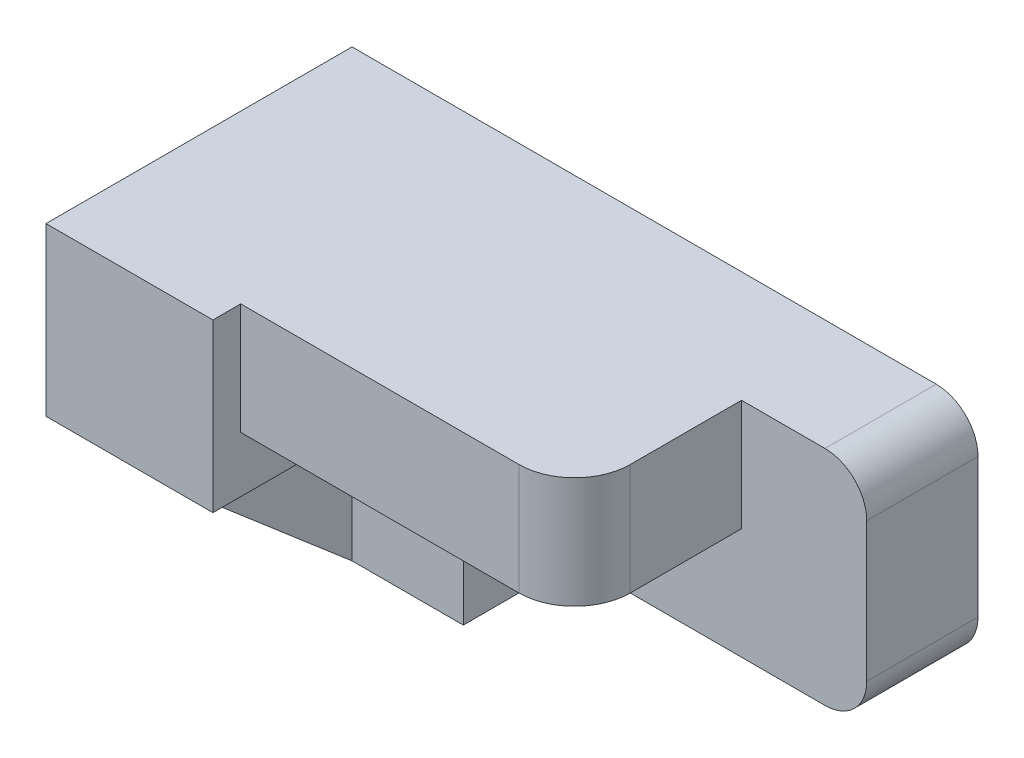
ISO-10303-21;
HEADER;
FILE_DESCRIPTION(('STEP AP214'),'2;1');
FILE_NAME('part.step','',(''),(''),'','','');
FILE_SCHEMA(('AUTOMOTIVE_DESIGN { 1 0 10303 214 1 1 1 1 }'));
ENDSEC;
DATA;
#1=APPLICATION_CONTEXT('core data for automotive mechanical design processes');
#2=APPLICATION_PROTOCOL_DEFINITION('international standard','automotive_design',2000,#1);
#3=PRODUCT_CONTEXT('',#1,'mechanical');
#4=PRODUCT('Part','Part','',(#3));
#5=PRODUCT_RELATED_PRODUCT_CATEGORY('part','',(#4));
#6=PRODUCT_DEFINITION_FORMATION('','',#4);
#7=PRODUCT_DEFINITION_CONTEXT('part definition',#1,'design');
#8=PRODUCT_DEFINITION('design','',#6,#7);
#9=PRODUCT_DEFINITION_SHAPE('','',#8);
#10=(LENGTH_UNIT() NAMED_UNIT(*) SI_UNIT(.MILLI.,.METRE.));
#11=(NAMED_UNIT(*) PLANE_ANGLE_UNIT() SI_UNIT($,.RADIAN.));
#12=(NAMED_UNIT(*) SI_UNIT($,.STERADIAN.) SOLID_ANGLE_UNIT());
#13=UNCERTAINTY_MEASURE_WITH_UNIT(LENGTH_MEASURE(1.E-05),#10,'distance_accuracy_value','');
#14=(GEOMETRIC_REPRESENTATION_CONTEXT(3) GLOBAL_UNCERTAINTY_ASSIGNED_CONTEXT((#13)) GLOBAL_UNIT_ASSIGNED_CONTEXT((#10,
#11,#12)) REPRESENTATION_CONTEXT('',''));
#15=CARTESIAN_POINT('',(0.,0.,0.));
#16=DIRECTION('',(0.,0.,1.));
#17=DIRECTION('',(1.,0.,0.));
#18=AXIS2_PLACEMENT_3D('',#15,#16,#17);
#19=CARTESIAN_POINT('',(20.,10.,55.));
#20=DIRECTION('',(0.,-0.759256602365297,0.650791373455968));
#21=DIRECTION('',(0.,-0.650791373455968,-0.759256602365297));
#22=AXIS2_PLACEMENT_3D('',#19,#20,#21);
#23=PLANE('',#22);
#24=DIRECTION('',(1.,0.,0.));
#25=VECTOR('',#24,1.);
#26=CARTESIAN_POINT('',(30.,10.,55.));
#27=LINE('',#26,#25);
#28=CARTESIAN_POINT('',(12.,10.,55.));
#29=VERTEX_POINT('',#28);
#30=CARTESIAN_POINT('',(20.,10.,55.));
#31=VERTEX_POINT('',#30);
#32=EDGE_CURVE('E68',#29,#31,#27,.T.);
#33=ORIENTED_EDGE('',*,*,#32,.F.);
#34=DIRECTION('',(0.,0.650791373455969,0.759256602365297));
#35=VECTOR('',#34,1.);
#36=CARTESIAN_POINT('',(12.,10.,55.));
#37=LINE('',#36,#35);
#38=CARTESIAN_POINT('',(12.,-20.,20.));
#39=VERTEX_POINT('',#38);
#40=EDGE_CURVE('E185',#39,#29,#37,.T.);
#41=ORIENTED_EDGE('',*,*,#40,.F.);
#42=DIRECTION('',(-1.,0.,0.));
#43=VECTOR('',#42,1.);
#44=CARTESIAN_POINT('',(20.,-20.,20.));
#45=LINE('',#44,#43);
#46=CARTESIAN_POINT('',(20.,-20.,20.));
#47=VERTEX_POINT('',#46);
#48=EDGE_CURVE('E202',#47,#39,#45,.T.);
#49=ORIENTED_EDGE('',*,*,#48,.F.);
#50=DIRECTION('',(0.,0.650791373455969,0.759256602365297));
#51=VECTOR('',#50,1.);
#52=CARTESIAN_POINT('',(20.,10.,55.));
#53=LINE('',#52,#51);
#54=EDGE_CURVE('E200',#47,#31,#53,.T.);
#55=ORIENTED_EDGE('',*,*,#54,.T.);
#56=EDGE_LOOP('',(#33,#41,#49,#55));
#57=FACE_BOUND('',#56,.T.);
#58=ADVANCED_FACE('F50',(#57),#23,.T.);
#59=CARTESIAN_POINT('',(105.,7.5,20.));
#60=DIRECTION('',(0.,0.,1.));
#61=DIRECTION('',(1.,0.,0.));
#62=AXIS2_PLACEMENT_3D('',#59,#60,#61);
#63=PLANE('',#62);
#64=DIRECTION('',(0.,-1.,0.));
#65=VECTOR('',#64,1.);
#66=CARTESIAN_POINT('',(20.,-20.,20.));
#67=LINE('',#66,#65);
#68=CARTESIAN_POINT('',(20.,10.,20.));
#69=VERTEX_POINT('',#68);
#70=EDGE_CURVE('E193',#69,#47,#67,.T.);
#71=ORIENTED_EDGE('',*,*,#70,.T.);
#72=DIRECTION('',(-1.,0.,0.));
#73=VECTOR('',#72,1.);
#74=CARTESIAN_POINT('',(0.,-20.,20.));
#75=LINE('',#74,#73);
#76=CARTESIAN_POINT('',(40.,-20.,20.));
#77=VERTEX_POINT('',#76);
#78=EDGE_CURVE('E268',#77,#47,#75,.T.);
#79=ORIENTED_EDGE('',*,*,#78,.F.);
#80=DIRECTION('',(0.,1.,0.));
#81=VECTOR('',#80,1.);
#82=CARTESIAN_POINT('',(40.,-20.,20.));
#83=LINE('',#82,#81);
#84=CARTESIAN_POINT('',(40.,0.,20.));
#85=VERTEX_POINT('',#84);
#86=EDGE_CURVE('E271',#77,#85,#83,.T.);
#87=ORIENTED_EDGE('',*,*,#86,.T.);
#88=DIRECTION('',(1.,0.,0.));
#89=VECTOR('',#88,1.);
#90=CARTESIAN_POINT('',(0.,0.,20.));
#91=LINE('',#90,#89);
#92=CARTESIAN_POINT('',(105.,0.,20.));
#93=VERTEX_POINT('',#92);
#94=EDGE_CURVE('E278',#85,#93,#91,.T.);
#95=ORIENTED_EDGE('',*,*,#94,.T.);
#96=CARTESIAN_POINT('',(105.,7.5,20.));
#97=DIRECTION('',(0.,0.,1.));
#98=DIRECTION('',(1.,0.,0.));
#99=AXIS2_PLACEMENT_3D('',#96,#97,#98);
#100=CIRCLE('',#99,7.5);
#101=CARTESIAN_POINT('',(112.5,7.5,20.));
#102=VERTEX_POINT('',#101);
#103=EDGE_CURVE('E285',#93,#102,#100,.T.);
#104=ORIENTED_EDGE('',*,*,#103,.T.);
#105=DIRECTION('',(0.,1.,0.));
#106=VECTOR('',#105,1.);
#107=CARTESIAN_POINT('',(112.5,32.5,20.));
#108=LINE('',#107,#106);
#109=CARTESIAN_POINT('',(112.5,32.5,20.));
#110=VERTEX_POINT('',#109);
#111=EDGE_CURVE('E281',#102,#110,#108,.T.);
#112=ORIENTED_EDGE('',*,*,#111,.T.);
#113=CARTESIAN_POINT('',(105.,32.5,20.));
#114=DIRECTION('',(0.,0.,1.));
#115=DIRECTION('',(1.,0.,0.));
#116=AXIS2_PLACEMENT_3D('',#113,#114,#115);
#117=CIRCLE('',#116,7.5);
#118=CARTESIAN_POINT('',(105.,40.,20.));
#119=VERTEX_POINT('',#118);
#120=EDGE_CURVE('E289',#110,#119,#117,.T.);
#121=ORIENTED_EDGE('',*,*,#120,.T.);
#122=DIRECTION('',(-1.,0.,0.));
#123=VECTOR('',#122,1.);
#124=CARTESIAN_POINT('',(0.,40.,20.));
#125=LINE('',#124,#123);
#126=CARTESIAN_POINT('',(90.,40.,20.));
#127=VERTEX_POINT('',#126);
#128=EDGE_CURVE('E286',#119,#127,#125,.T.);
#129=ORIENTED_EDGE('',*,*,#128,.T.);
#130=DIRECTION('',(0.,1.,0.));
#131=VECTOR('',#130,1.);
#132=CARTESIAN_POINT('',(90.,20.,20.));
#133=LINE('',#132,#131);
#134=CARTESIAN_POINT('',(90.,20.,20.));
#135=VERTEX_POINT('',#134);
#136=EDGE_CURVE('E231',#135,#127,#133,.T.);
#137=ORIENTED_EDGE('',*,*,#136,.F.);
#138=DIRECTION('',(1.,0.,0.));
#139=VECTOR('',#138,1.);
#140=CARTESIAN_POINT('',(0.,20.,20.));
#141=LINE('',#140,#139);
#142=CARTESIAN_POINT('',(30.,20.,20.));
#143=VERTEX_POINT('',#142);
#144=EDGE_CURVE('E217',#143,#135,#141,.T.);
#145=ORIENTED_EDGE('',*,*,#144,.F.);
#146=DIRECTION('',(0.,1.,0.));
#147=VECTOR('',#146,1.);
#148=CARTESIAN_POINT('',(30.,40.,20.));
#149=LINE('',#148,#147);
#150=CARTESIAN_POINT('',(30.,10.,20.));
#151=VERTEX_POINT('',#150);
#152=EDGE_CURVE('E243',#151,#143,#149,.T.);
#153=ORIENTED_EDGE('',*,*,#152,.F.);
#154=DIRECTION('',(1.,0.,0.));
#155=VECTOR('',#154,1.);
#156=CARTESIAN_POINT('',(30.,10.,20.));
#157=LINE('',#156,#155);
#158=EDGE_CURVE('E235',#69,#151,#157,.T.);
#159=ORIENTED_EDGE('',*,*,#158,.F.);
#160=EDGE_LOOP('',(#71,#79,#87,#95,#104,#112,#121,#129,#137,#145,#153,#159));
#161=FACE_BOUND('',#160,.T.);
#162=ADVANCED_FACE('F333',(#161),#63,.T.);
#163=CARTESIAN_POINT('',(0.,0.,20.));
#164=DIRECTION('',(0.,1.,0.));
#165=DIRECTION('',(0.,0.,1.));
#166=AXIS2_PLACEMENT_3D('',#163,#164,#165);
#167=PLANE('',#166);
#168=DIRECTION('',(0.,0.,1.));
#169=VECTOR('',#168,1.);
#170=CARTESIAN_POINT('',(40.,0.,20.));
#171=LINE('',#170,#169);
#172=CARTESIAN_POINT('',(40.,0.,0.));
#173=VERTEX_POINT('',#172);
#174=EDGE_CURVE('E257',#173,#85,#171,.T.);
#175=ORIENTED_EDGE('',*,*,#174,.F.);
#176=DIRECTION('',(1.,0.,0.));
#177=VECTOR('',#176,1.);
#178=CARTESIAN_POINT('',(0.,0.,0.));
#179=LINE('',#178,#177);
#180=CARTESIAN_POINT('',(105.,0.,0.));
#181=VERTEX_POINT('',#180);
#182=EDGE_CURVE('E294',#173,#181,#179,.T.);
#183=ORIENTED_EDGE('',*,*,#182,.T.);
#184=DIRECTION('',(0.,0.,-1.));
#185=VECTOR('',#184,1.);
#186=CARTESIAN_POINT('',(105.,0.,20.));
#187=LINE('',#186,#185);
#188=EDGE_CURVE('E11',#93,#181,#187,.T.);
#189=ORIENTED_EDGE('',*,*,#188,.F.);
#190=ORIENTED_EDGE('',*,*,#94,.F.);
#191=EDGE_LOOP('',(#175,#183,#189,#190));
#192=FACE_BOUND('',#191,.T.);
#193=ADVANCED_FACE('F342',(#192),#167,.F.);
#194=CARTESIAN_POINT('',(0.,40.,20.));
#195=DIRECTION('',(1.,0.,0.));
#196=DIRECTION('',(0.,0.,-1.));
#197=AXIS2_PLACEMENT_3D('',#194,#195,#196);
#198=PLANE('',#197);
#199=DIRECTION('',(0.,-1.,0.));
#200=VECTOR('',#199,1.);
#201=CARTESIAN_POINT('',(0.,-20.,20.));
#202=LINE('',#201,#200);
#203=CARTESIAN_POINT('',(0.,10.,20.));
#204=VERTEX_POINT('',#203);
#205=CARTESIAN_POINT('',(0.,-20.,20.));
#206=VERTEX_POINT('',#205);
#207=EDGE_CURVE('E189',#204,#206,#202,.T.);
#208=ORIENTED_EDGE('',*,*,#207,.F.);
#209=DIRECTION('',(0.,0.,-1.));
#210=VECTOR('',#209,1.);
#211=CARTESIAN_POINT('',(0.,10.,20.));
#212=LINE('',#211,#210);
#213=CARTESIAN_POINT('',(0.,10.,55.));
#214=VERTEX_POINT('',#213);
#215=EDGE_CURVE('E180',#214,#204,#212,.T.);
#216=ORIENTED_EDGE('',*,*,#215,.F.);
#217=DIRECTION('',(0.,-1.,0.));
#218=VECTOR('',#217,1.);
#219=CARTESIAN_POINT('',(0.,10.,55.));
#220=LINE('',#219,#218);
#221=CARTESIAN_POINT('',(0.,40.,55.));
#222=VERTEX_POINT('',#221);
#223=EDGE_CURVE('E239',#222,#214,#220,.T.);
#224=ORIENTED_EDGE('',*,*,#223,.F.);
#225=DIRECTION('',(0.,0.,-1.));
#226=VECTOR('',#225,1.);
#227=CARTESIAN_POINT('',(0.,40.,20.));
#228=LINE('',#227,#226);
#229=CARTESIAN_POINT('',(0.,40.,0.));
#230=VERTEX_POINT('',#229);
#231=EDGE_CURVE('E295',#222,#230,#228,.T.);
#232=ORIENTED_EDGE('',*,*,#231,.T.);
#233=DIRECTION('',(0.,-1.,0.));
#234=VECTOR('',#233,1.);
#235=CARTESIAN_POINT('',(0.,40.,0.));
#236=LINE('',#235,#234);
#237=CARTESIAN_POINT('',(0.,-20.,0.));
#238=VERTEX_POINT('',#237);
#239=EDGE_CURVE('E276',#230,#238,#236,.T.);
#240=ORIENTED_EDGE('',*,*,#239,.T.);
#241=DIRECTION('',(0.,0.,-1.));
#242=VECTOR('',#241,1.);
#243=CARTESIAN_POINT('',(0.,-20.,0.));
#244=LINE('',#243,#242);
#245=EDGE_CURVE('E261',#206,#238,#244,.T.);
#246=ORIENTED_EDGE('',*,*,#245,.F.);
#247=EDGE_LOOP('',(#208,#216,#224,#232,#240,#246));
#248=FACE_BOUND('',#247,.T.);
#249=ADVANCED_FACE('F47',(#248),#198,.F.);
#250=CARTESIAN_POINT('',(105.,7.5,20.));
#251=DIRECTION('',(0.,0.,-1.));
#252=DIRECTION('',(-1.,0.,0.));
#253=AXIS2_PLACEMENT_3D('',#250,#251,#252);
#254=CYLINDRICAL_SURFACE('',#253,7.5);
#255=CARTESIAN_POINT('',(105.,7.5,0.));
#256=DIRECTION('',(0.,0.,1.));
#257=DIRECTION('',(1.,0.,0.));
#258=AXIS2_PLACEMENT_3D('',#255,#256,#257);
#259=CIRCLE('',#258,7.5);
#260=CARTESIAN_POINT('',(112.5,7.5,0.));
#261=VERTEX_POINT('',#260);
#262=EDGE_CURVE('E297',#181,#261,#259,.T.);
#263=ORIENTED_EDGE('',*,*,#262,.T.);
#264=DIRECTION('',(0.,0.,-1.));
#265=VECTOR('',#264,1.);
#266=CARTESIAN_POINT('',(112.5,7.5,20.));
#267=LINE('',#266,#265);
#268=EDGE_CURVE('E54',#102,#261,#267,.T.);
#269=ORIENTED_EDGE('',*,*,#268,.F.);
#270=ORIENTED_EDGE('',*,*,#103,.F.);
#271=ORIENTED_EDGE('',*,*,#188,.T.);
#272=EDGE_LOOP('',(#263,#269,#270,#271));
#273=FACE_BOUND('',#272,.T.);
#274=ADVANCED_FACE('F338',(#273),#254,.T.);
#275=CARTESIAN_POINT('',(112.5,32.5,20.));
#276=DIRECTION('',(-1.,0.,0.));
#277=DIRECTION('',(0.,0.,1.));
#278=AXIS2_PLACEMENT_3D('',#275,#276,#277);
#279=PLANE('',#278);
#280=DIRECTION('',(0.,1.,0.));
#281=VECTOR('',#280,1.);
#282=CARTESIAN_POINT('',(112.5,32.5,0.));
#283=LINE('',#282,#281);
#284=CARTESIAN_POINT('',(112.5,32.5,0.));
#285=VERTEX_POINT('',#284);
#286=EDGE_CURVE('E298',#261,#285,#283,.T.);
#287=ORIENTED_EDGE('',*,*,#286,.T.);
#288=DIRECTION('',(0.,0.,-1.));
#289=VECTOR('',#288,1.);
#290=CARTESIAN_POINT('',(112.5,32.5,20.));
#291=LINE('',#290,#289);
#292=EDGE_CURVE('E306',#110,#285,#291,.T.);
#293=ORIENTED_EDGE('',*,*,#292,.F.);
#294=ORIENTED_EDGE('',*,*,#111,.F.);
#295=ORIENTED_EDGE('',*,*,#268,.T.);
#296=EDGE_LOOP('',(#287,#293,#294,#295));
#297=FACE_BOUND('',#296,.T.);
#298=ADVANCED_FACE('F312',(#297),#279,.F.);
#299=CARTESIAN_POINT('',(105.,32.5,20.));
#300=DIRECTION('',(0.,0.,-1.));
#301=DIRECTION('',(-1.,0.,0.));
#302=AXIS2_PLACEMENT_3D('',#299,#300,#301);
#303=CYLINDRICAL_SURFACE('',#302,7.5);
#304=CARTESIAN_POINT('',(105.,32.5,0.));
#305=DIRECTION('',(0.,0.,1.));
#306=DIRECTION('',(1.,0.,0.));
#307=AXIS2_PLACEMENT_3D('',#304,#305,#306);
#308=CIRCLE('',#307,7.5);
#309=CARTESIAN_POINT('',(105.,40.,0.));
#310=VERTEX_POINT('',#309);
#311=EDGE_CURVE('E296',#285,#310,#308,.T.);
#312=ORIENTED_EDGE('',*,*,#311,.T.);
#313=DIRECTION('',(0.,0.,-1.));
#314=VECTOR('',#313,1.);
#315=CARTESIAN_POINT('',(105.,40.,20.));
#316=LINE('',#315,#314);
#317=EDGE_CURVE('E303',#119,#310,#316,.T.);
#318=ORIENTED_EDGE('',*,*,#317,.F.);
#319=ORIENTED_EDGE('',*,*,#120,.F.);
#320=ORIENTED_EDGE('',*,*,#292,.T.);
#321=EDGE_LOOP('',(#312,#318,#319,#320));
#322=FACE_BOUND('',#321,.T.);
#323=ADVANCED_FACE('F330',(#322),#303,.T.);
#324=CARTESIAN_POINT('',(0.,40.,20.));
#325=DIRECTION('',(0.,-1.,0.));
#326=DIRECTION('',(0.,0.,-1.));
#327=AXIS2_PLACEMENT_3D('',#324,#325,#326);
#328=PLANE('',#327);
#329=DIRECTION('',(0.,0.,1.));
#330=VECTOR('',#329,1.);
#331=CARTESIAN_POINT('',(90.,40.,0.));
#332=LINE('',#331,#330);
#333=CARTESIAN_POINT('',(90.,40.,40.));
#334=VERTEX_POINT('',#333);
#335=EDGE_CURVE('E213',#127,#334,#332,.T.);
#336=ORIENTED_EDGE('',*,*,#335,.F.);
#337=ORIENTED_EDGE('',*,*,#128,.F.);
#338=ORIENTED_EDGE('',*,*,#317,.T.);
#339=DIRECTION('',(-1.,0.,0.));
#340=VECTOR('',#339,1.);
#341=CARTESIAN_POINT('',(0.,40.,0.));
#342=LINE('',#341,#340);
#343=EDGE_CURVE('E283',#310,#230,#342,.T.);
#344=ORIENTED_EDGE('',*,*,#343,.T.);
#345=ORIENTED_EDGE('',*,*,#231,.F.);
#346=DIRECTION('',(-1.,0.,0.));
#347=VECTOR('',#346,1.);
#348=CARTESIAN_POINT('',(0.,40.,55.));
#349=LINE('',#348,#347);
#350=CARTESIAN_POINT('',(30.,40.,55.));
#351=VERTEX_POINT('',#350);
#352=EDGE_CURVE('E250',#351,#222,#349,.T.);
#353=ORIENTED_EDGE('',*,*,#352,.F.);
#354=DIRECTION('',(0.,0.,-1.));
#355=VECTOR('',#354,1.);
#356=CARTESIAN_POINT('',(30.,40.,55.));
#357=LINE('',#356,#355);
#358=CARTESIAN_POINT('',(30.,40.,50.));
#359=VERTEX_POINT('',#358);
#360=EDGE_CURVE('E253',#351,#359,#357,.T.);
#361=ORIENTED_EDGE('',*,*,#360,.T.);
#362=DIRECTION('',(1.,0.,0.));
#363=VECTOR('',#362,1.);
#364=CARTESIAN_POINT('',(0.,40.,50.));
#365=LINE('',#364,#363);
#366=CARTESIAN_POINT('',(80.,40.,50.));
#367=VERTEX_POINT('',#366);
#368=EDGE_CURVE('E208',#359,#367,#365,.T.);
#369=ORIENTED_EDGE('',*,*,#368,.T.);
#370=CARTESIAN_POINT('',(80.,40.,40.));
#371=DIRECTION('',(0.,1.,0.));
#372=DIRECTION('',(0.,0.,1.));
#373=AXIS2_PLACEMENT_3D('',#370,#371,#372);
#374=CIRCLE('',#373,10.);
#375=EDGE_CURVE('E223',#367,#334,#374,.T.);
#376=ORIENTED_EDGE('',*,*,#375,.T.);
#377=EDGE_LOOP('',(#336,#337,#338,#344,#345,#353,#361,#369,#376));
#378=FACE_BOUND('',#377,.T.);
#379=ADVANCED_FACE('F335',(#378),#328,.F.);
#380=CARTESIAN_POINT('',(105.,7.5,0.));
#381=DIRECTION('',(0.,0.,1.));
#382=DIRECTION('',(1.,0.,0.));
#383=AXIS2_PLACEMENT_3D('',#380,#381,#382);
#384=PLANE('',#383);
#385=ORIENTED_EDGE('',*,*,#239,.F.);
#386=ORIENTED_EDGE('',*,*,#343,.F.);
#387=ORIENTED_EDGE('',*,*,#311,.F.);
#388=ORIENTED_EDGE('',*,*,#286,.F.);
#389=ORIENTED_EDGE('',*,*,#262,.F.);
#390=ORIENTED_EDGE('',*,*,#182,.F.);
#391=DIRECTION('',(0.,1.,0.));
#392=VECTOR('',#391,1.);
#393=CARTESIAN_POINT('',(40.,-20.,0.));
#394=LINE('',#393,#392);
#395=CARTESIAN_POINT('',(40.,-20.,0.));
#396=VERTEX_POINT('',#395);
#397=EDGE_CURVE('E277',#396,#173,#394,.T.);
#398=ORIENTED_EDGE('',*,*,#397,.F.);
#399=DIRECTION('',(1.,0.,0.));
#400=VECTOR('',#399,1.);
#401=CARTESIAN_POINT('',(40.,-20.,0.));
#402=LINE('',#401,#400);
#403=EDGE_CURVE('E262',#238,#396,#402,.T.);
#404=ORIENTED_EDGE('',*,*,#403,.F.);
#405=EDGE_LOOP('',(#385,#386,#387,#388,#389,#390,#398,#404));
#406=FACE_BOUND('',#405,.T.);
#407=ADVANCED_FACE('F323',(#406),#384,.F.);
#408=CARTESIAN_POINT('',(40.,-20.,20.));
#409=DIRECTION('',(-1.,0.,0.));
#410=DIRECTION('',(0.,0.,1.));
#411=AXIS2_PLACEMENT_3D('',#408,#409,#410);
#412=PLANE('',#411);
#413=ORIENTED_EDGE('',*,*,#174,.T.);
#414=ORIENTED_EDGE('',*,*,#86,.F.);
#415=DIRECTION('',(0.,0.,1.));
#416=VECTOR('',#415,1.);
#417=CARTESIAN_POINT('',(40.,-20.,20.));
#418=LINE('',#417,#416);
#419=EDGE_CURVE('E266',#396,#77,#418,.T.);
#420=ORIENTED_EDGE('',*,*,#419,.F.);
#421=ORIENTED_EDGE('',*,*,#397,.T.);
#422=EDGE_LOOP('',(#413,#414,#420,#421));
#423=FACE_BOUND('',#422,.T.);
#424=ADVANCED_FACE('F350',(#423),#412,.F.);
#425=CARTESIAN_POINT('',(0.,-20.,0.));
#426=DIRECTION('',(0.,1.,0.));
#427=DIRECTION('',(0.,0.,1.));
#428=AXIS2_PLACEMENT_3D('',#425,#426,#427);
#429=PLANE('',#428);
#430=ORIENTED_EDGE('',*,*,#245,.T.);
#431=ORIENTED_EDGE('',*,*,#403,.T.);
#432=ORIENTED_EDGE('',*,*,#419,.T.);
#433=ORIENTED_EDGE('',*,*,#78,.T.);
#434=ORIENTED_EDGE('',*,*,#48,.T.);
#435=DIRECTION('',(-1.,0.,0.));
#436=VECTOR('',#435,1.);
#437=CARTESIAN_POINT('',(12.,-20.,20.));
#438=LINE('',#437,#436);
#439=EDGE_CURVE('E182',#39,#206,#438,.T.);
#440=ORIENTED_EDGE('',*,*,#439,.T.);
#441=EDGE_LOOP('',(#430,#431,#432,#433,#434,#440));
#442=FACE_BOUND('',#441,.T.);
#443=ADVANCED_FACE('F348',(#442),#429,.F.);
#444=CARTESIAN_POINT('',(30.,10.,55.));
#445=DIRECTION('',(0.,1.,0.));
#446=DIRECTION('',(0.,0.,1.));
#447=AXIS2_PLACEMENT_3D('',#444,#445,#446);
#448=PLANE('',#447);
#449=CARTESIAN_POINT('',(30.,10.,55.));
#450=VERTEX_POINT('',#449);
#451=EDGE_CURVE('E245',#31,#450,#27,.T.);
#452=ORIENTED_EDGE('',*,*,#451,.F.);
#453=DIRECTION('',(0.,0.,-1.));
#454=VECTOR('',#453,1.);
#455=CARTESIAN_POINT('',(20.,10.,20.));
#456=LINE('',#455,#454);
#457=EDGE_CURVE('E205',#31,#69,#456,.T.);
#458=ORIENTED_EDGE('',*,*,#457,.T.);
#459=ORIENTED_EDGE('',*,*,#158,.T.);
#460=DIRECTION('',(0.,0.,-1.));
#461=VECTOR('',#460,1.);
#462=CARTESIAN_POINT('',(30.,10.,55.));
#463=LINE('',#462,#461);
#464=EDGE_CURVE('E260',#450,#151,#463,.T.);
#465=ORIENTED_EDGE('',*,*,#464,.F.);
#466=EDGE_LOOP('',(#452,#458,#459,#465));
#467=FACE_BOUND('',#466,.T.);
#468=ADVANCED_FACE('F377',(#467),#448,.F.);
#469=CARTESIAN_POINT('',(30.,40.,55.));
#470=DIRECTION('',(-1.,0.,0.));
#471=DIRECTION('',(0.,0.,1.));
#472=AXIS2_PLACEMENT_3D('',#469,#470,#471);
#473=PLANE('',#472);
#474=DIRECTION('',(0.,0.,-1.));
#475=VECTOR('',#474,1.);
#476=CARTESIAN_POINT('',(30.,20.,0.));
#477=LINE('',#476,#475);
#478=CARTESIAN_POINT('',(30.,20.,50.));
#479=VERTEX_POINT('',#478);
#480=EDGE_CURVE('E219',#479,#143,#477,.T.);
#481=ORIENTED_EDGE('',*,*,#480,.F.);
#482=DIRECTION('',(0.,1.,0.));
#483=VECTOR('',#482,1.);
#484=CARTESIAN_POINT('',(30.,20.,50.));
#485=LINE('',#484,#483);
#486=EDGE_CURVE('E226',#479,#359,#485,.T.);
#487=ORIENTED_EDGE('',*,*,#486,.T.);
#488=ORIENTED_EDGE('',*,*,#360,.F.);
#489=DIRECTION('',(0.,1.,0.));
#490=VECTOR('',#489,1.);
#491=CARTESIAN_POINT('',(30.,40.,55.));
#492=LINE('',#491,#490);
#493=EDGE_CURVE('E247',#450,#351,#492,.T.);
#494=ORIENTED_EDGE('',*,*,#493,.F.);
#495=ORIENTED_EDGE('',*,*,#464,.T.);
#496=ORIENTED_EDGE('',*,*,#152,.T.);
#497=EDGE_LOOP('',(#481,#487,#488,#494,#495,#496));
#498=FACE_BOUND('',#497,.T.);
#499=ADVANCED_FACE('F362',(#498),#473,.F.);
#500=CARTESIAN_POINT('',(0.,0.,55.));
#501=DIRECTION('',(0.,0.,-1.));
#502=DIRECTION('',(-1.,0.,0.));
#503=AXIS2_PLACEMENT_3D('',#500,#501,#502);
#504=PLANE('',#503);
#505=ORIENTED_EDGE('',*,*,#223,.T.);
#506=EDGE_CURVE('E244',#214,#29,#27,.T.);
#507=ORIENTED_EDGE('',*,*,#506,.T.);
#508=ORIENTED_EDGE('',*,*,#32,.T.);
#509=ORIENTED_EDGE('',*,*,#451,.T.);
#510=ORIENTED_EDGE('',*,*,#493,.T.);
#511=ORIENTED_EDGE('',*,*,#352,.T.);
#512=EDGE_LOOP('',(#505,#507,#508,#509,#510,#511));
#513=FACE_BOUND('',#512,.T.);
#514=ADVANCED_FACE('F351',(#513),#504,.F.);
#515=CARTESIAN_POINT('',(0.,20.,50.));
#516=DIRECTION('',(0.,0.,1.));
#517=DIRECTION('',(1.,0.,0.));
#518=AXIS2_PLACEMENT_3D('',#515,#516,#517);
#519=PLANE('',#518);
#520=ORIENTED_EDGE('',*,*,#368,.F.);
#521=ORIENTED_EDGE('',*,*,#486,.F.);
#522=DIRECTION('',(1.,0.,0.));
#523=VECTOR('',#522,1.);
#524=CARTESIAN_POINT('',(0.,20.,50.));
#525=LINE('',#524,#523);
#526=CARTESIAN_POINT('',(80.,20.,50.));
#527=VERTEX_POINT('',#526);
#528=EDGE_CURVE('E207',#479,#527,#525,.T.);
#529=ORIENTED_EDGE('',*,*,#528,.T.);
#530=DIRECTION('',(0.,1.,0.));
#531=VECTOR('',#530,1.);
#532=CARTESIAN_POINT('',(80.,20.,50.));
#533=LINE('',#532,#531);
#534=EDGE_CURVE('E225',#527,#367,#533,.T.);
#535=ORIENTED_EDGE('',*,*,#534,.T.);
#536=EDGE_LOOP('',(#520,#521,#529,#535));
#537=FACE_BOUND('',#536,.T.);
#538=ADVANCED_FACE('F364',(#537),#519,.T.);
#539=CARTESIAN_POINT('',(90.,20.,0.));
#540=DIRECTION('',(-1.,0.,0.));
#541=DIRECTION('',(0.,0.,1.));
#542=AXIS2_PLACEMENT_3D('',#539,#540,#541);
#543=PLANE('',#542);
#544=ORIENTED_EDGE('',*,*,#335,.T.);
#545=DIRECTION('',(0.,1.,0.));
#546=VECTOR('',#545,1.);
#547=CARTESIAN_POINT('',(90.,20.,40.));
#548=LINE('',#547,#546);
#549=CARTESIAN_POINT('',(90.,20.,40.));
#550=VERTEX_POINT('',#549);
#551=EDGE_CURVE('E237',#550,#334,#548,.T.);
#552=ORIENTED_EDGE('',*,*,#551,.F.);
#553=DIRECTION('',(0.,0.,1.));
#554=VECTOR('',#553,1.);
#555=CARTESIAN_POINT('',(90.,20.,0.));
#556=LINE('',#555,#554);
#557=EDGE_CURVE('E216',#135,#550,#556,.T.);
#558=ORIENTED_EDGE('',*,*,#557,.F.);
#559=ORIENTED_EDGE('',*,*,#136,.T.);
#560=EDGE_LOOP('',(#544,#552,#558,#559));
#561=FACE_BOUND('',#560,.T.);
#562=ADVANCED_FACE('F373',(#561),#543,.F.);
#563=CARTESIAN_POINT('',(80.,20.,40.));
#564=DIRECTION('',(0.,1.,0.));
#565=DIRECTION('',(0.,0.,1.));
#566=AXIS2_PLACEMENT_3D('',#563,#564,#565);
#567=CYLINDRICAL_SURFACE('',#566,10.);
#568=ORIENTED_EDGE('',*,*,#375,.F.);
#569=ORIENTED_EDGE('',*,*,#534,.F.);
#570=CARTESIAN_POINT('',(80.,20.,40.));
#571=DIRECTION('',(0.,1.,0.));
#572=DIRECTION('',(0.,0.,1.));
#573=AXIS2_PLACEMENT_3D('',#570,#571,#572);
#574=CIRCLE('',#573,10.);
#575=EDGE_CURVE('E215',#527,#550,#574,.T.);
#576=ORIENTED_EDGE('',*,*,#575,.T.);
#577=ORIENTED_EDGE('',*,*,#551,.T.);
#578=EDGE_LOOP('',(#568,#569,#576,#577));
#579=FACE_BOUND('',#578,.T.);
#580=ADVANCED_FACE('F369',(#579),#567,.T.);
#581=CARTESIAN_POINT('',(0.,20.,0.));
#582=DIRECTION('',(0.,1.,0.));
#583=DIRECTION('',(0.,0.,1.));
#584=AXIS2_PLACEMENT_3D('',#581,#582,#583);
#585=PLANE('',#584);
#586=ORIENTED_EDGE('',*,*,#528,.F.);
#587=ORIENTED_EDGE('',*,*,#480,.T.);
#588=ORIENTED_EDGE('',*,*,#144,.T.);
#589=ORIENTED_EDGE('',*,*,#557,.T.);
#590=ORIENTED_EDGE('',*,*,#575,.F.);
#591=EDGE_LOOP('',(#586,#587,#588,#589,#590));
#592=FACE_BOUND('',#591,.T.);
#593=ADVANCED_FACE('F374',(#592),#585,.F.);
#594=CARTESIAN_POINT('',(20.,0.,0.));
#595=DIRECTION('',(1.,0.,0.));
#596=DIRECTION('',(0.,0.,-1.));
#597=AXIS2_PLACEMENT_3D('',#594,#595,#596);
#598=PLANE('',#597);
#599=ORIENTED_EDGE('',*,*,#70,.F.);
#600=ORIENTED_EDGE('',*,*,#457,.F.);
#601=ORIENTED_EDGE('',*,*,#54,.F.);
#602=EDGE_LOOP('',(#599,#600,#601));
#603=FACE_BOUND('',#602,.T.);
#604=ADVANCED_FACE('F385',(#603),#598,.T.);
#605=CARTESIAN_POINT('',(12.,10.,20.));
#606=DIRECTION('',(0.,1.,0.));
#607=DIRECTION('',(0.,0.,1.));
#608=AXIS2_PLACEMENT_3D('',#605,#606,#607);
#609=PLANE('',#608);
#610=ORIENTED_EDGE('',*,*,#215,.T.);
#611=DIRECTION('',(-1.,0.,0.));
#612=VECTOR('',#611,1.);
#613=CARTESIAN_POINT('',(12.,10.,20.));
#614=LINE('',#613,#612);
#615=CARTESIAN_POINT('',(12.,10.,20.));
#616=VERTEX_POINT('',#615);
#617=EDGE_CURVE('E174',#616,#204,#614,.T.);
#618=ORIENTED_EDGE('',*,*,#617,.F.);
#619=DIRECTION('',(0.,0.,-1.));
#620=VECTOR('',#619,1.);
#621=CARTESIAN_POINT('',(12.,10.,20.));
#622=LINE('',#621,#620);
#623=EDGE_CURVE('E177',#29,#616,#622,.T.);
#624=ORIENTED_EDGE('',*,*,#623,.F.);
#625=ORIENTED_EDGE('',*,*,#506,.F.);
#626=EDGE_LOOP('',(#610,#618,#624,#625));
#627=FACE_BOUND('',#626,.T.);
#628=ADVANCED_FACE('F171',(#627),#609,.F.);
#629=CARTESIAN_POINT('',(12.,-20.,20.));
#630=DIRECTION('',(0.,0.,-1.));
#631=DIRECTION('',(-1.,0.,0.));
#632=AXIS2_PLACEMENT_3D('',#629,#630,#631);
#633=PLANE('',#632);
#634=ORIENTED_EDGE('',*,*,#207,.T.);
#635=ORIENTED_EDGE('',*,*,#439,.F.);
#636=DIRECTION('',(0.,-1.,0.));
#637=VECTOR('',#636,1.);
#638=CARTESIAN_POINT('',(12.,-20.,20.));
#639=LINE('',#638,#637);
#640=EDGE_CURVE('E65',#616,#39,#639,.T.);
#641=ORIENTED_EDGE('',*,*,#640,.F.);
#642=ORIENTED_EDGE('',*,*,#617,.T.);
#643=EDGE_LOOP('',(#634,#635,#641,#642));
#644=FACE_BOUND('',#643,.T.);
#645=ADVANCED_FACE('F184',(#644),#633,.F.);
#646=CARTESIAN_POINT('',(12.,0.,0.));
#647=DIRECTION('',(-1.,0.,0.));
#648=DIRECTION('',(0.,0.,1.));
#649=AXIS2_PLACEMENT_3D('',#646,#647,#648);
#650=PLANE('',#649);
#651=ORIENTED_EDGE('',*,*,#623,.T.);
#652=ORIENTED_EDGE('',*,*,#640,.T.);
#653=ORIENTED_EDGE('',*,*,#40,.T.);
#654=EDGE_LOOP('',(#651,#652,#653));
#655=FACE_BOUND('',#654,.T.);
#656=ADVANCED_FACE('F188',(#655),#650,.T.);
#657=CLOSED_SHELL('',(#58,#162,#193,#249,#274,#298,#323,#379,#407,#424,#443,#468,#499,#514,#538,
#562,#580,#593,#604,#628,#645,#656));
#658=MANIFOLD_SOLID_BREP('B2',#657);
#659=ADVANCED_BREP_SHAPE_REPRESENTATION('',(#18,#658),#14);
#660=SHAPE_DEFINITION_REPRESENTATION(#9,#659);
ENDSEC;
END-ISO-10303-21;
